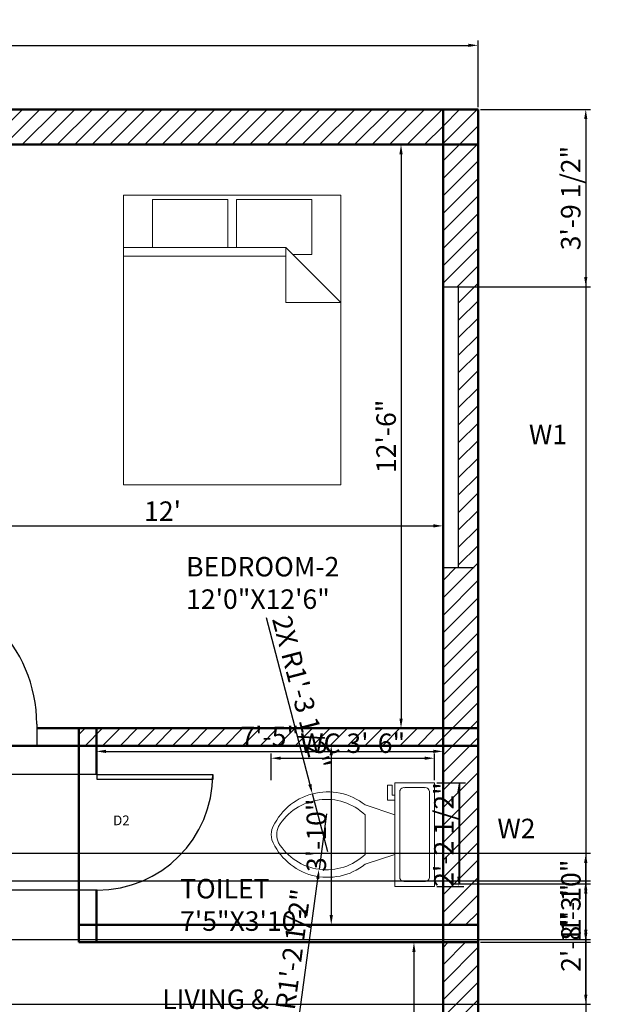
# Model space of a CAD drawing. Units: millimetres. Extents: x 2600 to 3013, y 1440 to 2066.
# Tile 4 of 4: x 2864 to 3013, y 1768 to 2021. Entities that reach past the tile are written whole.
import ezdxf

# ---------------------------------------------------------------- set-up
doc = ezdxf.new("R2010")
doc.units = ezdxf.units.MM
for name, color, linetype, lineweight in [('A-AREA-IDEN', 130, 'Continuous', 25), ('A-FLOR-FIXT', 160, 'Continuous', 18), ('A-WALL-PATT', 90, 'Continuous', 13), ('dimensions', 50, 'Continuous', 18), ('doors', 200, 'Continuous', 25), ('furniture', 160, 'Continuous', 18), ('text', 130, 'Continuous', 18), ('walls', 90, 'Continuous', 50), ('windows', 30, 'Continuous', 25)]:
    doc.layers.add(name, color=color, linetype=linetype, lineweight=lineweight)
doc.styles.get("Standard").update_dxf_attribs({"font": 'arial.ttf'})
doc.dimstyles.new('ISO-25', dxfattribs={"dimtxt": 5, "dimasz": 2.5, "dimexe": 1.25, "dimexo": 0.625, "dimtad": 1, "dimdec": 1, "dimlunit": 3, "dimtxsty": 'Standard', "dimcen": 2.5, "dimadec": 0, "dimazin": 0, "dimtfac": 1, "dimtdec": 1, "dimtmove": 0, "dimatfit": 3, "dimfxl": 1, "dimarcsym": 0})

# ---------------------------------------------------------------- blocks, each defined once
blk = doc.blocks.new('*U2')
for p, q in [((0, 0), (0, -6)), ((40, 0), (40, -6))]:
    blk.add_line(p, q)
blk.add_lwpolyline([(0, 0), (0, 40), (1.75, 40), (1.75, 0)], close=True)
blk.add_arc((0, 0), 40, 0, 90)
blk = doc.blocks.new('*U4')
for p, q in [((0, 4), (0, 0)), ((36, 4), (36, 0)), ((0, 2), (36, 2))]:
    blk.add_line(p, q)
blk = doc.blocks.new('*U6')
for p, q in [((0, 4), (0, 0)), ((36, 4), (36, 0)), ((0, 2), (36, 2))]:
    blk.add_line(p, q)
blk = doc.blocks.new('Toilet - top')
for p, q in [((9.5, -6), (9.5, -2)), ((-10, -8.5), (-8, -8.5)), ((-10, -9.5), (-10, -8.5)), ((-7, -9.5), (-10, -9.5)), ((-8, -8.5), (-8, -8)), ((-7, -8), (-7, -9.5)), ((-4, -8), (-6, -14)), ((4, -8), (6, -14)), ((4, -14), (-4, -14))]:
    blk.add_line(p, q)
blk.add_lwpolyline([(10.5, -8), (10.5, 0), (-10.5, 0), (-10.5, -8)], close=True)
for points in [[(8.5, -1), (-8.5, -1)], [(-9.5, -2), (-9.5, -6)], [(-8.5, -7), (8.5, -7)]]:
    blk.add_lwpolyline(points)
for centre, radius, start, end in [((-8.62, -1.88), 0.884, 81.8699, 188.1301), ((8.62, -1.88), 0.884, 351.8699, 98.1301), ((-8.62, -6.12), 0.884, 171.8699, 278.1301), ((8.62, -6.12), 0.884, 261.8699, 8.1301), ((3.52, -21.58), 12.17, 141.4691, 247.9714), ((4.2, -21.82), 11.33, 136.3677, 238.9468), ((-3.52, -21.58), 12.17, 292.0284, 38.5307), ((-4.2, -21.82), 11.33, 301.053, 43.6321), ((0, -27.88), 4, 245.7318, 294.2682), ((0, -29), 4, 254.8605, 285.1395)]:
    blk.add_arc(centre, radius, start, end)
blk = doc.blocks.new('Bed - Queen')
for p, q in [((0, -80.00003), (0, 0)), ((0, 0), (59.99999, 0)), ((59.99999, 0), (59.99999, -80.00003)), ((7.99999, -1.2), (28.79998, -1.2)), ((7.99999, -14.4), (7.99999, -1.2)), ((28.79998, -1.2), (28.79998, -14.4)), ((31.19999, -1.2), (51.99999, -1.2)), ((31.19999, -14.4), (31.19999, -1.2)), ((51.99999, -1.2), (51.99999, -16.4)), ((0, -14.4), (44.8, -14.4)), ((59.99999, -29.6), (44.8, -14.4)), ((44.8, -14.4), (44.8, -29.6)), ((44.8, -16.8), (0, -16.8)), ((51.99999, -16.4), (46.79936, -16.4)), ((44.8, -29.6), (59.99999, -29.6)), ((59.99999, -80.00003), (0, -80.00003))]:
    blk.add_line(p, q)
blk = doc.blocks.new('*D12')
at = {"layer": 'Defpoints', "color": 0, "transparency": 16777216}
for p in [(2828.26, 1889.98), (2972.26, 1890.68), (2972.26, 1890.68)]:
    blk.add_point(p, dxfattribs=at)
at = {"layer": 'dimensions', "color": 0, "lineweight": -2, "transparency": 16777216}
for p, q in [((2828.26, 1890.6), (2828.26, 1891.93)), ((2830.76, 1890.68), (2969.76, 1890.68)), ((2972.26, 1891.3), (2972.26, 1891.93))]:
    blk.add_line(p, q, dxfattribs=at)
at = {"layer": 'dimensions', "color": 0, "transparency": 16777216}
for points in [[(2830.76, 1891.1), (2830.76, 1890.26), (2828.26, 1890.68)], [(2969.76, 1891.1), (2969.76, 1890.26), (2972.26, 1890.68)]]:
    blk.add_solid(points, dxfattribs=at)
at = {"layer": 'dimensions', "color": 0, "transparency": 16777216, "insert": (2900.26, 1893.81), "char_height": 5, "attachment_point": 5}
blk.add_mtext("12'", dxfattribs=at)
blk = doc.blocks.new('*D13')
at = {"layer": 'Defpoints', "color": 0, "transparency": 16777216}
for p in [(2961.48, 1988.68), (2961.48, 1838.68), (2961.48, 1838.68)]:
    blk.add_point(p, dxfattribs=at)
at = {"layer": 'dimensions', "color": 0, "lineweight": -2, "transparency": 16777216}
for p, q in [((2962.11, 1988.68), (2962.73, 1988.68)), ((2961.48, 1986.18), (2961.48, 1841.18)), ((2962.11, 1838.68), (2962.73, 1838.68))]:
    blk.add_line(p, q, dxfattribs=at)
at = {"layer": 'dimensions', "color": 0, "transparency": 16777216}
for points in [[(2961.06, 1986.18), (2961.9, 1986.18), (2961.48, 1988.68)], [(2961.06, 1841.18), (2961.9, 1841.18), (2961.48, 1838.68)]]:
    blk.add_solid(points, dxfattribs=at)
at = {"layer": 'dimensions', "color": 0, "transparency": 16777216, "insert": (2958.3, 1913.68), "char_height": 5, "attachment_point": 5, "rotation": 90}
blk.add_mtext('12\'-6"', dxfattribs=at)
blk = doc.blocks.new('*D16')
at = {"layer": 'Defpoints', "color": 0, "transparency": 16777216}
for p in [(2951.12, 1834.18), (2943.56, 1788.18), (2951.12, 1788.18)]:
    blk.add_point(p, dxfattribs=at)
at = {"layer": 'dimensions', "color": 0, "lineweight": -2, "transparency": 16777216}
for p, q in [((2950.5, 1834.18), (2942.31, 1834.18)), ((2943.56, 1831.68), (2943.56, 1790.68)), ((2950.5, 1788.18), (2942.31, 1788.18))]:
    blk.add_line(p, q, dxfattribs=at)
at = {"layer": 'dimensions', "color": 0, "transparency": 16777216}
for points in [[(2943.14, 1831.68), (2943.98, 1831.68), (2943.56, 1834.18)], [(2943.14, 1790.68), (2943.98, 1790.68), (2943.56, 1788.18)]]:
    blk.add_solid(points, dxfattribs=at)
at = {"layer": 'dimensions', "color": 0, "transparency": 16777216, "insert": (2940.38, 1811.18), "char_height": 5, "attachment_point": 5, "rotation": 90}
blk.add_mtext('3\'-10"', dxfattribs=at)
blk = doc.blocks.new('*D17')
at = {"layer": 'Defpoints', "color": 0, "transparency": 16777216}
for p in [(2883.26, 1832.74), (2972.26, 1832.74), (2972.26, 1832.74)]:
    blk.add_point(p, dxfattribs=at)
at = {"layer": 'dimensions', "color": 0, "lineweight": -2, "transparency": 16777216}
for p, q in [((2883.26, 1833.37), (2883.26, 1833.99)), ((2885.76, 1832.74), (2969.76, 1832.74)), ((2972.26, 1833.37), (2972.26, 1833.99))]:
    blk.add_line(p, q, dxfattribs=at)
at = {"layer": 'dimensions', "color": 0, "transparency": 16777216}
for points in [[(2885.76, 1833.16), (2885.76, 1832.32), (2883.26, 1832.74)], [(2969.76, 1833.16), (2969.76, 1832.32), (2972.26, 1832.74)]]:
    blk.add_solid(points, dxfattribs=at)
at = {"layer": 'dimensions', "color": 0, "transparency": 16777216, "insert": (2927.76, 1835.91), "char_height": 5, "attachment_point": 5}
blk.add_mtext('7\'-5"', dxfattribs=at)
blk = doc.blocks.new('*D21')
at = {"layer": 'Defpoints', "color": 0, "transparency": 16777216}
for p in [(2964.8, 1783.68), (2964.8, 1611.68), (2964.8, 1611.68)]:
    blk.add_point(p, dxfattribs=at)
at = {"layer": 'dimensions', "color": 0, "lineweight": -2, "transparency": 16777216}
for p, q in [((2965.42, 1783.68), (2966.05, 1783.68)), ((2964.8, 1781.18), (2964.8, 1614.18)), ((2965.42, 1611.68), (2966.05, 1611.68))]:
    blk.add_line(p, q, dxfattribs=at)
at = {"layer": 'dimensions', "color": 0, "transparency": 16777216}
for points in [[(2964.38, 1781.18), (2965.21, 1781.18), (2964.8, 1783.68)], [(2964.38, 1614.18), (2965.21, 1614.18), (2964.8, 1611.68)]]:
    blk.add_solid(points, dxfattribs=at)
at = {"layer": 'dimensions', "color": 0, "transparency": 16777216, "insert": (2961.66, 1697.68), "char_height": 5, "attachment_point": 5, "rotation": 90}
blk.add_mtext('14\'-4"', dxfattribs=at)
blk = doc.blocks.new('*D27')
at = {"layer": 'Defpoints', "color": 0, "transparency": 16777216}
for p in [(2981.26, 2014.15), (2694.76, 1997.68), (2981.26, 1997.68)]:
    blk.add_point(p, dxfattribs=at)
at = {"layer": 'dimensions', "color": 0, "lineweight": -2, "transparency": 16777216}
for p, q in [((2694.76, 1998.3), (2694.76, 2015.4)), ((2697.26, 2014.15), (2978.76, 2014.15)), ((2981.26, 1998.3), (2981.26, 2015.4))]:
    blk.add_line(p, q, dxfattribs=at)
at = {"layer": 'dimensions', "color": 0, "transparency": 16777216}
for points in [[(2697.26, 2014.57), (2697.26, 2013.74), (2694.76, 2014.15)], [(2978.76, 2014.57), (2978.76, 2013.74), (2981.26, 2014.15)]]:
    blk.add_solid(points, dxfattribs=at)
at = {"layer": 'dimensions', "color": 0, "transparency": 16777216, "insert": (2838.01, 2017.33), "char_height": 5, "attachment_point": 5}
blk.add_mtext('23\'-10.5"', dxfattribs=at)
blk = doc.blocks.new('*D33')
at = {"layer": 'Defpoints', "color": 0, "transparency": 16777216}
for p in [(2970.03, 1830.98), (2928.1, 1824.69), (2970.03, 1824.69)]:
    blk.add_point(p, dxfattribs=at)
at = {"layer": 'dimensions', "color": 0, "lineweight": -2, "transparency": 16777216}
for p, q in [((2928.1, 1825.31), (2928.1, 1832.23)), ((2970.03, 1825.31), (2970.03, 1832.23)), ((2930.6, 1830.98), (2967.53, 1830.98))]:
    blk.add_line(p, q, dxfattribs=at)
at = {"layer": 'dimensions', "color": 0, "transparency": 16777216}
for points in [[(2930.6, 1831.39), (2930.6, 1830.56), (2928.1, 1830.98)], [(2967.53, 1831.39), (2967.53, 1830.56), (2970.03, 1830.98)]]:
    blk.add_solid(points, dxfattribs=at)
at = {"layer": 'dimensions', "color": 0, "transparency": 16777216, "insert": (2949.07, 1834.19), "char_height": 5, "attachment_point": 5}
blk.add_mtext('WC 3\'-6"', dxfattribs=at)
blk = doc.blocks.new('*D34')
at = {"layer": 'Defpoints', "color": 0, "transparency": 16777216}
for p in [(2970.03, 1824.69), (2970.03, 1798.03), (2976.33, 1798.03)]:
    blk.add_point(p, dxfattribs=at)
at = {"layer": 'dimensions', "color": 0, "lineweight": -2, "transparency": 16777216}
for p, q in [((2970.66, 1824.69), (2977.58, 1824.69)), ((2976.33, 1822.19), (2976.33, 1800.53)), ((2970.66, 1798.03), (2977.58, 1798.03))]:
    blk.add_line(p, q, dxfattribs=at)
at = {"layer": 'dimensions', "color": 0, "transparency": 16777216}
for points in [[(2975.91, 1822.19), (2976.74, 1822.19), (2976.33, 1824.69)], [(2975.91, 1800.53), (2976.74, 1800.53), (2976.33, 1798.03)]]:
    blk.add_solid(points, dxfattribs=at)
at = {"layer": 'dimensions', "color": 0, "transparency": 16777216, "insert": (2973.12, 1811.36), "char_height": 5, "attachment_point": 5, "rotation": 90}
blk.add_mtext('2\'-2 1/2"', dxfattribs=at)
blk = doc.blocks.new('*D35')
at = {"layer": 'Defpoints', "color": 0, "transparency": 16777216}
for p in [(2981.26, 1997.68), (2875.72, 1472.18), (3008.91, 1472.18)]:
    blk.add_point(p, dxfattribs=at)
at = {"layer": 'dimensions', "color": 0, "lineweight": -2, "transparency": 16777216}
for p, q in [((2981.88, 1997.68), (3010.16, 1997.68)), ((3008.91, 1995.18), (3008.91, 1474.68)), ((2876.34, 1472.18), (3010.16, 1472.18))]:
    blk.add_line(p, q, dxfattribs=at)
at = {"layer": 'dimensions', "color": 0, "transparency": 16777216}
for points in [[(3008.49, 1995.18), (3009.32, 1995.18), (3008.91, 1997.68)], [(3008.49, 1474.68), (3009.32, 1474.68), (3008.91, 1472.18)]]:
    blk.add_solid(points, dxfattribs=at)
at = {"layer": 'dimensions', "color": 0, "transparency": 16777216, "insert": (3005.69, 1734.93), "char_height": 5, "attachment_point": 5, "rotation": 90}
blk.add_mtext('43\'-9 1/2"', dxfattribs=at)
blk = doc.blocks.new('*D44')
at = {"layer": 'Defpoints', "color": 0, "transparency": 16777216}
for p in [(2883.26, 1826.8), (2667.11, 1797.08), (2883.26, 1797.08)]:
    blk.add_point(p, dxfattribs=at)
at = {"layer": 'dimensions', "color": 0, "lineweight": -2, "transparency": 16777216}
for p, q in [((2882.63, 1826.8), (2665.86, 1826.8)), ((2667.11, 1824.3), (2667.11, 1799.58)), ((2882.63, 1797.08), (2665.86, 1797.08))]:
    blk.add_line(p, q, dxfattribs=at)
at = {"layer": 'dimensions', "color": 0, "transparency": 16777216}
for points in [[(2666.69, 1824.3), (2667.52, 1824.3), (2667.11, 1826.8)], [(2666.69, 1799.58), (2667.52, 1799.58), (2667.11, 1797.08)]]:
    blk.add_solid(points, dxfattribs=at)
at = {"layer": 'dimensions', "color": 0, "transparency": 16777216, "insert": (2663.9, 1811.94), "char_height": 5, "attachment_point": 5, "rotation": 90}
blk.add_mtext('2\'-5 1/2"', dxfattribs=at)
blk = doc.blocks.new('*D47')
at = {"layer": 'Defpoints', "color": 0, "transparency": 16777216}
for p in [(2780.26, 1799.5), (3008.91, 1799.5), (2780.26, 1767.75)]:
    blk.add_point(p, dxfattribs=at)
at = {"layer": 'dimensions', "color": 0, "lineweight": -2, "transparency": 16777216}
for p, q in [((2780.88, 1799.5), (3010.16, 1799.5)), ((3008.91, 1770.25), (3008.91, 1797)), ((2780.88, 1767.75), (3010.16, 1767.75))]:
    blk.add_line(p, q, dxfattribs=at)
at = {"layer": 'dimensions', "color": 0, "transparency": 16777216}
for points in [[(3008.49, 1797), (3009.32, 1797), (3008.91, 1799.5)], [(3008.49, 1770.25), (3009.32, 1770.25), (3008.91, 1767.75)]]:
    blk.add_solid(points, dxfattribs=at)
at = {"layer": 'dimensions', "color": 0, "transparency": 16777216, "insert": (3005.73, 1783.63), "char_height": 5, "attachment_point": 5, "rotation": 90}
blk.add_mtext('2\'-8"', dxfattribs=at)
blk = doc.blocks.new('*D49')
at = {"layer": 'Defpoints', "color": 0, "transparency": 16777216}
for p in [(2719.39, 1806.57), (3008.91, 1806.57), (2719.39, 1784.43)]:
    blk.add_point(p, dxfattribs=at)
at = {"layer": 'dimensions', "color": 0, "lineweight": -2, "transparency": 16777216}
for p, q in [((2720.01, 1806.57), (3010.16, 1806.57)), ((3008.91, 1786.93), (3008.91, 1804.07)), ((2720.01, 1784.43), (3010.16, 1784.43))]:
    blk.add_line(p, q, dxfattribs=at)
at = {"layer": 'dimensions', "color": 0, "transparency": 16777216}
for points in [[(3008.49, 1804.07), (3009.32, 1804.07), (3008.91, 1806.57)], [(3008.49, 1786.93), (3009.32, 1786.93), (3008.91, 1784.43)]]:
    blk.add_solid(points, dxfattribs=at)
at = {"layer": 'dimensions', "color": 0, "transparency": 16777216, "insert": (3005.73, 1795.5), "char_height": 5, "attachment_point": 5, "rotation": 90}
blk.add_mtext('1\'-10"', dxfattribs=at)
blk = doc.blocks.new('*D51')
at = {"layer": 'Defpoints', "color": 0, "transparency": 16777216}
for p in [(2981.26, 1997.68), (2976.27, 1952.13), (3008.91, 1952.13)]:
    blk.add_point(p, dxfattribs=at)
at = {"layer": 'dimensions', "color": 0, "lineweight": -2, "transparency": 16777216}
for p, q in [((2981.88, 1997.68), (3010.16, 1997.68)), ((3008.91, 1995.18), (3008.91, 1954.63)), ((2976.89, 1952.13), (3010.16, 1952.13))]:
    blk.add_line(p, q, dxfattribs=at)
at = {"layer": 'dimensions', "color": 0, "transparency": 16777216}
for points in [[(3008.49, 1995.18), (3009.32, 1995.18), (3008.91, 1997.68)], [(3008.49, 1954.63), (3009.32, 1954.63), (3008.91, 1952.13)]]:
    blk.add_solid(points, dxfattribs=at)
at = {"layer": 'dimensions', "color": 0, "transparency": 16777216, "insert": (3005.69, 1974.9), "char_height": 5, "attachment_point": 5, "rotation": 90}
blk.add_mtext('3\'-9 1/2"', dxfattribs=at)
blk = doc.blocks.new('*D53')
at = {"layer": 'Defpoints', "color": 0, "transparency": 16777216}
for p in [(2976.59, 1798.67), (3008.91, 1798.67), (2981.26, 1783.68)]:
    blk.add_point(p, dxfattribs=at)
at = {"layer": 'dimensions', "color": 0, "lineweight": -2, "transparency": 16777216}
for p, q in [((2977.22, 1798.67), (3010.16, 1798.67)), ((3008.91, 1786.18), (3008.91, 1796.17)), ((2981.88, 1783.68), (3010.16, 1783.68))]:
    blk.add_line(p, q, dxfattribs=at)
at = {"layer": 'dimensions', "color": 0, "transparency": 16777216}
for points in [[(3008.49, 1796.17), (3009.32, 1796.17), (3008.91, 1798.67)], [(3008.49, 1786.18), (3009.32, 1786.18), (3008.91, 1783.68)]]:
    blk.add_solid(points, dxfattribs=at)
at = {"layer": 'dimensions', "color": 0, "transparency": 16777216, "insert": (3005.73, 1791.18), "char_height": 5, "attachment_point": 5, "rotation": 90}
blk.add_mtext('1\'-3"', dxfattribs=at)
blk = doc.blocks.new('*D61')
at = {"layer": 'Defpoints', "color": 0, "transparency": 16777216}
for p in [(2938.72, 1821.83), (2942.65, 1806.89)]:
    blk.add_point(p, dxfattribs=at)
at = {"layer": 'dimensions', "color": 0, "lineweight": -2, "transparency": 16777216}
for p, q in [((2926.83, 1867.1), (2938.09, 1824.25)), ((2942.65, 1806.89), (2938.72, 1821.83))]:
    blk.add_line(p, q, dxfattribs=at)
at = {"layer": 'dimensions', "color": 0, "transparency": 16777216}
blk.add_solid([(2938.49, 1824.35), (2937.68, 1824.14), (2938.72, 1821.83)], dxfattribs=at)
at = {"layer": 'dimensions', "color": 0, "transparency": 16777216, "insert": (2935.25, 1847.7), "char_height": 5, "attachment_point": 5, "rotation": 284.7218}
blk.add_mtext('2X R1\'-3 1/2"', dxfattribs=at)
blk = doc.blocks.new('*D62')
at = {"layer": 'Defpoints', "color": 0, "transparency": 16777216}
for p in [(2942.35, 1816.69), (2940.43, 1802.44)]:
    blk.add_point(p, dxfattribs=at)
at = {"layer": 'dimensions', "color": 0, "lineweight": -2, "transparency": 16777216}
for p, q in [((2942.35, 1816.69), (2940.43, 1802.44)), ((2934.19, 1756.05), (2940.1, 1799.96))]:
    blk.add_line(p, q, dxfattribs=at)
at = {"layer": 'dimensions', "color": 0, "transparency": 16777216}
blk.add_solid([(2939.68, 1800.02), (2940.51, 1799.91), (2940.43, 1802.44)], dxfattribs=at)
at = {"layer": 'dimensions', "color": 0, "transparency": 16777216, "insert": (2933.8, 1777.2), "char_height": 5, "attachment_point": 5, "rotation": 82.3419}
blk.add_mtext('2X R1\'-2 1/2"', dxfattribs=at)

msp = doc.modelspace()

# ---------------------------------------------------------------- hatches: boundary and pattern name
at = {"layer": 'A-WALL-PATT'}
h = msp.add_hatch(dxfattribs=at)
h.set_pattern_fill('ANSI31', color=256)
h.paths.add_polyline_path([(2972.26, 1997.68), (2828.26, 1997.68), (2828.26, 1988.68), (2972.26, 1988.68)])
h.paths.add_polyline_path([(2823.76, 1997.68), (2703.76, 1997.68), (2703.76, 1988.68), (2823.76, 1988.68)])
h.paths.add_polyline_path([(2828.26, 1997.68), (2823.76, 1997.68), (2823.76, 1988.68), (2828.26, 1988.68)])
h.paths.add_polyline_path([(2703.76, 1997.68), (2694.76, 1997.68), (2694.76, 1988.68), (2703.76, 1988.68)])
h.paths.add_polyline_path([(2703.76, 1988.68), (2694.76, 1988.68), (2694.76, 1958.65), (2698.77, 1958.65), (2698.77, 1886.48), (2694.76, 1886.48), (2694.76, 1838.68), (2703.76, 1838.68)])
h.paths.add_polyline_path([(2703.76, 1733.68), (2694.76, 1733.68), (2694.76, 1612.68), (2703.76, 1612.68)])
h.paths.add_polyline_path([(2703.76, 1608.18), (2694.76, 1608.18), (2694.76, 1506.18), (2703.76, 1506.18)])
h.paths.add_polyline_path([(2703.76, 1612.68), (2694.76, 1612.68), (2694.76, 1608.18), (2703.76, 1608.18)])
h.paths.add_polyline_path([(2823.76, 1612.68), (2703.76, 1612.68), (2703.76, 1608.18), (2823.76, 1608.18)])
h.paths.add_polyline_path([(2972.26, 1611.68), (2869.05, 1611.68, -0.005663), (2869.06, 1610.86), (2869.06, 1607.18), (2972.26, 1607.18)])
h.paths.add_polyline_path([(2981.26, 1607.18), (2972.26, 1607.18), (2972.26, 1506.18), (2981.26, 1506.18)])
h.paths.add_polyline_path([(2981.26, 1611.68), (2972.26, 1611.68), (2972.26, 1607.18), (2981.26, 1607.18)])
h.paths.add_polyline_path([(2828.26, 1569.75), (2824.68, 1569.8, -0.006355), (2823.76, 1569.82), (2823.76, 1506.18), (2828.26, 1506.18)])
h.paths.add_polyline_path([(2828.26, 1733.68), (2823.76, 1733.68), (2823.76, 1612.68), (2828.26, 1612.68)])
h.paths.add_polyline_path([(2981.26, 1783.68), (2972.26, 1783.68), (2972.26, 1611.68), (2981.26, 1611.68)])
h.paths.add_polyline_path([(2972.26, 1838.68), (2883.26, 1838.68), (2883.26, 1834.18), (2972.26, 1834.18)])
h.paths.add_polyline_path([(2981.26, 1838.68), (2972.26, 1838.68), (2972.26, 1834.18), (2981.26, 1834.18)])
h.paths.add_polyline_path([(2981.26, 1834.18), (2972.26, 1834.18), (2972.26, 1788.18), (2981.26, 1788.18)])
h.paths.add_polyline_path([(2981.26, 1988.68), (2972.26, 1988.68), (2972.26, 1952.13), (2976.27, 1952.13), (2976.27, 1879.95), (2972.26, 1879.95), (2972.26, 1838.68), (2981.26, 1838.68)])
h.paths.add_polyline_path([(2828.26, 1988.68), (2823.76, 1988.68), (2823.76, 1838.68), (2828.26, 1838.68)])
h.paths.add_polyline_path([(2780.26, 1834.18), (2775.76, 1834.18), (2775.76, 1799.5), (2780.26, 1799.5)])
h.paths.add_polyline_path([(2775.76, 1838.68), (2703.76, 1838.68), (2703.76, 1834.18), (2775.76, 1834.18)])
h.paths.add_polyline_path([(2780.26, 1838.68), (2775.76, 1838.68), (2775.76, 1834.18), (2780.26, 1834.18)])
h.paths.add_polyline_path([(2828.26, 1838.68), (2823.76, 1838.68), (2823.76, 1834.18), (2828.26, 1834.18)])
h.paths.add_polyline_path([(2883.26, 1838.68), (2878.76, 1838.68), (2878.76, 1834.18), (2883.26, 1834.18)])
h.paths.add_polyline_path([(2886.68, 1812.39), (2892.39, 1812.39), (2892.39, 1817.54), (2886.68, 1817.54)], flags=9)
h = msp.add_hatch(dxfattribs=at)
h.set_pattern_fill('ANSI31', color=256)
h.paths.add_polyline_path([(2703.76, 1834.18), (2694.76, 1834.18), (2694.76, 1738.18), (2703.76, 1738.18)])
h.paths.add_polyline_path([(2780.26, 1767.75), (2775.76, 1767.75), (2775.76, 1738.18), (2780.26, 1738.18)])
h.paths.add_polyline_path([(2972.26, 1506.18), (2868.8, 1506.18, -0.033203), (2869.12, 1501.37), (2869.12, 1497.18), (2972.26, 1497.18)])
h.paths.add_polyline_path([(2981.26, 1506.18), (2972.26, 1506.18), (2972.26, 1497.18), (2981.26, 1497.18)])
h.paths.add_polyline_path([(2823.76, 1506.18), (2703.76, 1506.18), (2703.76, 1497.18), (2823.76, 1497.18)])
h.paths.add_polyline_path([(2828.26, 1506.18), (2823.76, 1506.18), (2823.76, 1497.18), (2828.26, 1497.18)])
h.paths.add_polyline_path([(2832.8, 1506.18), (2828.26, 1506.18), (2828.26, 1497.18), (2832.8, 1497.18), (2832.8, 1501.37)])
h.paths.add_polyline_path([(2703.76, 1506.18), (2694.76, 1506.18), (2694.76, 1497.18), (2703.76, 1497.18)])
h.paths.add_polyline_path([(2981.26, 1997.68), (2972.26, 1997.68), (2972.26, 1988.68), (2981.26, 1988.68)])

# ---------------------------------------------------------------- linework, layer by layer
at = {"layer": 'walls'}
for p, q in [((2694.76, 1997.68), (2981.26, 1997.68)), ((2972.26, 1997.68), (2972.26, 1783.68)), ((2972.26, 1497.18), (2972.26, 1997.68)), ((2981.26, 1997.68), (2981.26, 1783.68)), ((2981.26, 1497.18), (2981.26, 1997.68)), ((2694.76, 1988.68), (2981.26, 1988.68)), ((2867.96, 1838.68), (2981.26, 1838.68)), ((2878.76, 1838.68), (2878.76, 1783.68)), ((2883.26, 1838.68), (2883.26, 1826.8)), ((2694.76, 1834.18), (2981.26, 1834.18)), ((2883.26, 1797.08), (2883.26, 1783.68)), ((2878.76, 1788.18), (2981.26, 1788.18)), ((2878.76, 1783.68), (2981.26, 1783.68))]:
    msp.add_line(p, q, dxfattribs=at)

# ---------------------------------------------------------------- block references
at = {"layer": 'A-FLOR-FIXT', "xscale": 1.269113081783838, "yscale": 1.269113081783838, "zscale": 1.269113081783838, "rotation": 270}
msp.add_blockref('Toilet - top', (2970.03, 1811.36), dxfattribs=at)
at = {"layer": 'doors', "xscale": 0.9079361683412358, "yscale": 0.9079361683412358, "zscale": 0.9079361683412358}
msp.add_blockref('*U2', (2831.64, 1839.73), dxfattribs=at)
at = {"layer": 'doors', "xscale": 0.7430263520936538, "yscale": 0.7430263520936538, "zscale": 0.7430263520936538, "rotation": 270}
msp.add_blockref('*U2', (2883.44, 1826.8), dxfattribs=at)
at = {"layer": 'furniture', "xscale": 0.9302566542625909, "yscale": 0.9302566542625909, "zscale": 0.9302566542625909}
msp.add_blockref('Bed - Queen', (2890.2, 1975.64), dxfattribs=at)
at = {"layer": 'windows', "rotation": 90}
for name, p, xscale, yscale, zscale in [('*U6', (2980.28, 1879.95), 2.004851231759801, 2.004851231759801, 2.004851231759801), ('*U4', (2978.04, 1798.67), 0.7216899638288952, 0.7216899638288952, 0.7216899638288952)]:
    msp.add_blockref(name, p, dxfattribs=dict(at, xscale=xscale, yscale=yscale, zscale=zscale))

# ---------------------------------------------------------------- texts
at = {"layer": 'A-AREA-IDEN', "char_height": 5, "attachment_point": 1}
for s, width, insert in [('BEDROOM-2\\P12\'0"X12\'6"', 38.6129, (2906.31, 1882.69)), ('TOILET\\P7\'5"X3\'10"', 19.4519, (2904.76, 1799.96)), ('LIVING & DINNING', 32.2605, (2900.18, 1771.56))]:
    msp.add_mtext_dynamic_manual_height_columns(s, width=width, gutter_width=12.5, heights=[0], dxfattribs=dict(at, insert=insert))
at = {"layer": 'text', "attachment_point": 1}
for s, width, insert, char_height in [('W1', 7.8518, (2994.32, 1916.67), 5), ('D2', 8.0594, (2887.57, 1816.26), 2.5), ('W2', 7.0233, (2986.22, 1815.43), 5)]:
    msp.add_mtext_dynamic_manual_height_columns(s, width=width, gutter_width=12.5, heights=[0], dxfattribs=dict(at, insert=insert, char_height=char_height))

# ---------------------------------------------------------------- dimensions: what is measured, and where the dimension line sits
at = {"layer": 'dimensions'}
for base, p1, p2, picture, middle in [((2981.26, 2014.15), (2694.76, 1997.68), (2981.26, 1997.68), '*D27', (2838.01, 2017.33)), ((2972.26, 1890.68), (2828.26, 1889.98), (2972.26, 1890.68), '*D12', (2900.26, 1893.81)), ((2972.26, 1832.74), (2883.26, 1832.74), (2972.26, 1832.74), '*D17', (2927.76, 1835.91))]:
    dim = msp.add_linear_dim(base=base, p1=p1, p2=p2, dimstyle='ISO-25', override={"dimclrd": 0, "dimclre": 0, "dimclrt": 0}, dxfattribs=at)
    dim.commit()
    dim.dimension.update_dxf_attribs({"geometry": picture, "text_midpoint": middle})
for base, p1, p2, angle, override, picture, middle in [((3008.91, 1472.18), (2981.26, 1997.68), (2875.72, 1472.18), 90, {"dimdec": 1, "dimlfac": 1, "dimrnd": 0, "dimzin": 1, "dimdsep": 46, "dimlunit": 4, "dimfrac": 2}, '*D35', (3005.69, 1734.93)), ((3008.9057, 1952.1252), (2981.2557, 1997.6793), (2976.2654, 1952.1252), 90, {"dimdec": 1, "dimlfac": 1, "dimrnd": 0, "dimzin": 1, "dimdsep": 46, "dimlunit": 4, "dimfrac": 2}, '*D51', (3005.6938, 1974.9023)), ((2961.48, 1838.68), (2961.48, 1988.68), (2961.48, 1838.68), 90, {"dimclrd": 0, "dimclre": 0, "dimclrt": 0}, '*D13', (2958.3, 1913.68)), ((2943.56, 1788.18), (2951.12, 1834.18), (2951.12, 1788.18), 90, {"dimclrd": 0, "dimclre": 0, "dimclrt": 0}, '*D16', (2940.38, 1811.18)), ((2667.11, 1797.08), (2883.26, 1826.8), (2883.26, 1797.08), 90, {"dimdec": 1, "dimlfac": 1, "dimrnd": 0, "dimzin": 1, "dimdsep": 46, "dimlunit": 4, "dimfrac": 2}, '*D44', (2663.9, 1811.94)), ((2976.33, 1798.03), (2970.03, 1824.69), (2970.03, 1798.03), 270, {"dimdec": 1, "dimlfac": 1, "dimrnd": 0, "dimzin": 1, "dimdsep": 46, "dimlunit": 4, "dimfrac": 2}, '*D34', (2973.12, 1811.36)), ((3008.91, 1806.57), (2719.39, 1784.43), (2719.39, 1806.57), 90, {"dimdec": 1, "dimlfac": 1, "dimrnd": 0, "dimzin": 1, "dimdsep": 46, "dimlunit": 4, "dimfrac": 2}, '*D49', (3005.73, 1795.5)), ((3008.9057, 1799.5016), (2780.2557, 1767.7507), (2780.2557, 1799.5016), 90, {"dimdec": 1, "dimlfac": 1, "dimrnd": 0, "dimzin": 1, "dimdsep": 46, "dimlunit": 4, "dimfrac": 2}, '*D47', (3005.7279, 1783.6262)), ((3008.91, 1798.67), (2981.26, 1783.68), (2976.59, 1798.67), 90, {"dimdec": 1, "dimlfac": 1, "dimrnd": 0, "dimzin": 1, "dimdsep": 46, "dimlunit": 4, "dimfrac": 2}, '*D53', (3005.73, 1791.18)), ((2964.8, 1611.68), (2964.8, 1783.68), (2964.8, 1611.68), 90, {"dimclrd": 0, "dimclre": 0, "dimclrt": 0}, '*D21', (2961.66, 1697.68))]:
    dim = msp.add_linear_dim(base=base, p1=p1, p2=p2, angle=angle, dimstyle='ISO-25', override=override, dxfattribs=at)
    dim.commit()
    dim.dimension.update_dxf_attribs({"geometry": picture, "text_midpoint": middle})
for center, mpoint, picture, middle in [((2942.65, 1806.89), (2938.72, 1821.83), '*D61', (2935.25, 1847.7)), ((2942.35, 1816.69), (2940.43, 1802.44), '*D62', (2933.8, 1777.2))]:
    dim = msp.add_radius_dim(center=center, mpoint=mpoint, text='2X <>', dimstyle='ISO-25', override={"dimdec": 1, "dimlfac": 1, "dimrnd": 0, "dimzin": 1, "dimdsep": 46, "dimlunit": 4, "dimfrac": 2}, dxfattribs=at)
    dim.commit()
    dim.dimension.update_dxf_attribs({"geometry": picture, "text_midpoint": middle})
dim = msp.add_linear_dim(base=(2970.03, 1830.98), p1=(2928.1, 1824.69), p2=(2970.03, 1824.69), text='WC <>', dimstyle='ISO-25', override={"dimdec": 1, "dimlfac": 1, "dimrnd": 0, "dimzin": 1, "dimdsep": 46, "dimlunit": 4, "dimfrac": 2}, dxfattribs=at)
dim.commit()
dim.dimension.update_dxf_attribs({"geometry": '*D33', "text_midpoint": (2949.07, 1834.19)})

doc.saveas('drawing.dxf')
